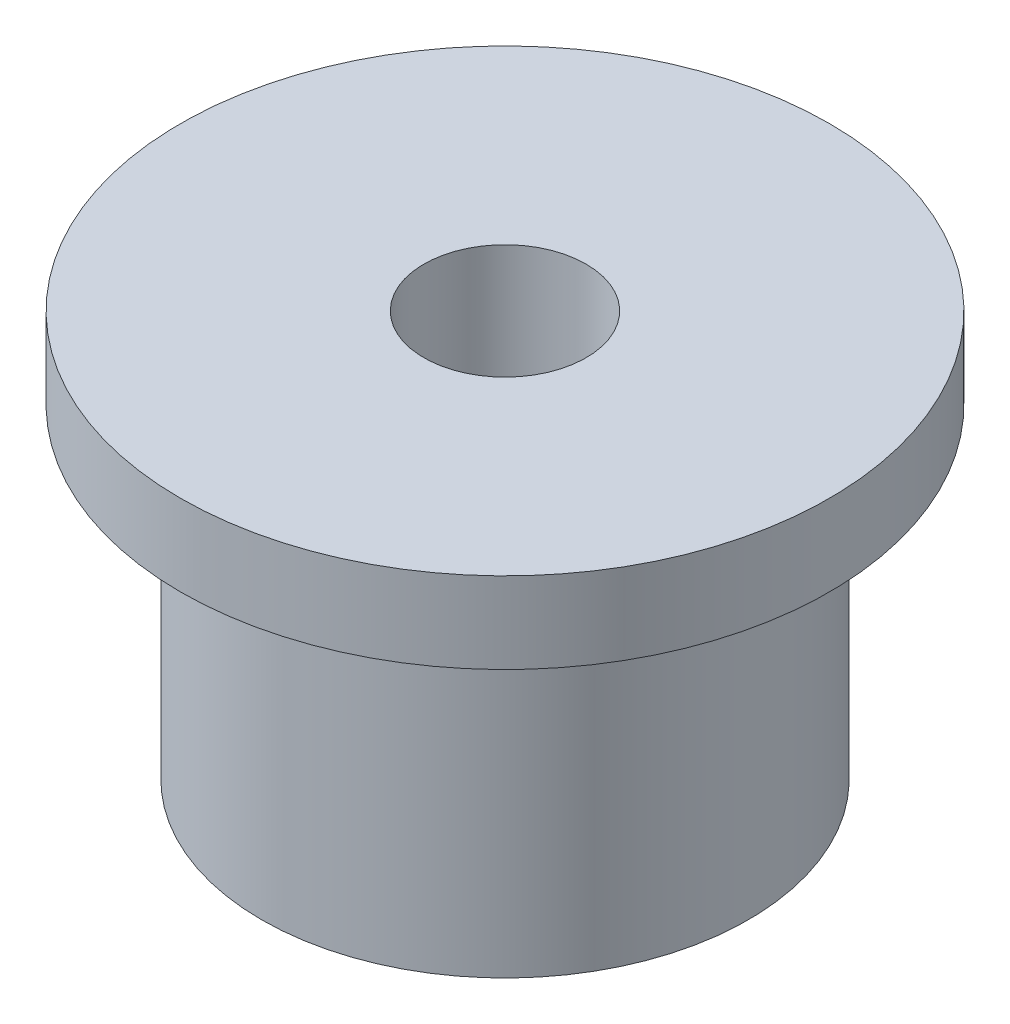
SolidWorks part; units mm, degrees
material "Cast Alloy Steel"
ref_plane "Front Plane" through (0, 0, 0) normal (0, 0, 1) x (1, 0, 0)
ref_plane "Top Plane" through (0, 0, 0) normal (0, 1, 0) x (1, 0, 0)
ref_plane "Right Plane" through (0, 0, 0) normal (1, 0, 0) x (0, 0, -1)
sketch "Bushing Half-Section Profile" plane through (0, 0, 0) normal (1, 0, 0) x (0, 0, -1)
  line L0 (25, 0) -> (25, 125)
  line L1 (25, 125) -> (100, 125)
  line L2 (100, 125) -> (100, 100)
  line L3 (100, 100) -> (75, 100)
  line L4 (75, 100) -> (75, 0)
  line L5 (75, 0) -> (25, 0)
  line L6 (0, 0) -> (0, 125) construction
  dimension "D1" = 25
  dimension "D2" = 75
  dimension "D3" = 100
  dimension "D4" = 25
  dimension "D5" = 125
revolve "Flanged Bushing Body" add sketch "Bushing Half-Section Profile" angle 360 about L6
